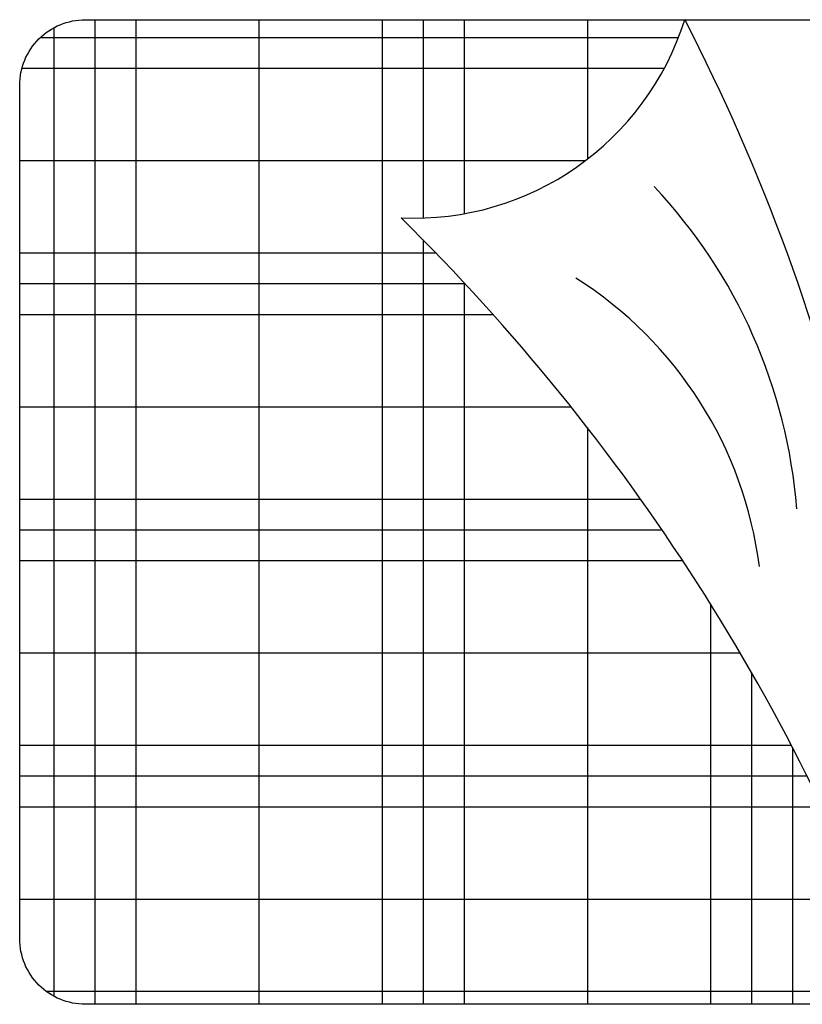
# Model space of a CAD drawing. Units: inches. Extents: x 3064 to 19385, y 846 to 15425.
# Tile 13 of 108: x 3711 to 3758, y 1034 to 1093. Entities that reach past the tile are written whole.
import ezdxf

# ---------------------------------------------------------------- set-up
doc = ezdxf.new("R2010")
doc.units = ezdxf.units.IN
doc.layers.add('A-FLOR-FIXT', color=9, linetype='Continuous', lineweight=18)
doc.layers.add('BLOCK', color=6, linetype='Continuous')

# ---------------------------------------------------------------- blocks, each defined once
blk = doc.blocks.new('*X5')
at = {"color": 0}
for p, q in [((276.598, 451.25), (280.51, 451.25)), ((275.455, 450.625), (280.51, 450.625)), ((274.411, 450), (280.51, 450)), ((265.51, 448.125), (267.634, 448.125)), ((271.723, 448.125), (280.51, 448.125)), ((265.51, 446.25), (268.465, 446.25)), ((269.519, 446.25), (280.51, 446.25)), ((265.51, 445.625), (268.531, 445.625)), ((268.866, 445.625), (280.51, 445.625)), ((265.51, 445), (280.51, 445)), ((265.51, 443.125), (280.51, 443.125)), ((265.51, 441.25), (280.51, 441.25)), ((265.51, 440.625), (280.51, 440.625)), ((265.634, 440), (280.386, 440))]:
    blk.add_line(p, q, dxfattribs=at)
blk = doc.blocks.new('*X6')
at = {"color": 0}
for p, q in [((280.312, 439.886), (280.312, 452.896)), ((278.906, 439.482), (278.906, 452.338)), ((277.5, 439.482), (277.5, 451.702)), ((277.031, 439.482), (277.031, 451.471)), ((276.562, 439.482), (276.562, 451.231)), ((275.156, 439.482), (275.156, 450.451)), ((273.75, 439.482), (273.75, 449.576)), ((265.781, 439.797), (265.781, 449.511)), ((266.25, 439.517), (266.25, 449.296)), ((273.281, 439.482), (273.281, 449.261)), ((272.812, 439.482), (272.812, 448.934)), ((267.656, 439.482), (267.656, 448.095)), ((271.406, 439.482), (271.406, 447.876)), ((270, 439.482), (270, 446.689)), ((269.531, 439.482), (269.531, 446.262)), ((269.062, 439.482), (269.062, 445.817))]:
    blk.add_line(p, q, dxfattribs=at)
blk = doc.blocks.new('A$C52E67D0D')
at = {"layer": 'BLOCK'}
blk.add_lwpolyline([(1901, 0), (601, 0, -0.414214), (501, 100), (501, 1700, -0.414214), (601, 1800), (1901, 1800, -0.414214), (2001, 1700), (2001, 100, -0.414214)], format="xyb", close=True, dxfattribs=at)
for centre, radius, start, end in [((1888.6, -1664.5), 3015.3, 87.8642, 117.4001), ((3101, -1685.8), 3227.7, 109.926, 135.3977), ((1308.8, 377.9), 807.6, 94.4436, 133.2788), ((1410.8, 520.2), 610.8, 97.2157, 147.6656), ((371.4, 600.4), 432, 357.3792, 72.5379)]:
    blk.add_arc(centre, radius, start, end, dxfattribs=at)
at = {"layer": 'BLOCK', "xscale": 100, "yscale": 100, "zscale": 100}
for name in ['*X6', '*X5']:
    blk.add_blockref(name, (-26050, -43948.2), dxfattribs=at)

msp = doc.modelspace()

# ---------------------------------------------------------------- block references
at = {"layer": 'A-FLOR-FIXT', "xscale": 0.039370099999992, "yscale": 0.039370099999992, "zscale": 0.039370099999992, "rotation": 270}
msp.add_blockref('A$C52E67D0D', (3711.493, 1112.592), dxfattribs=at)

doc.saveas('drawing.dxf')
